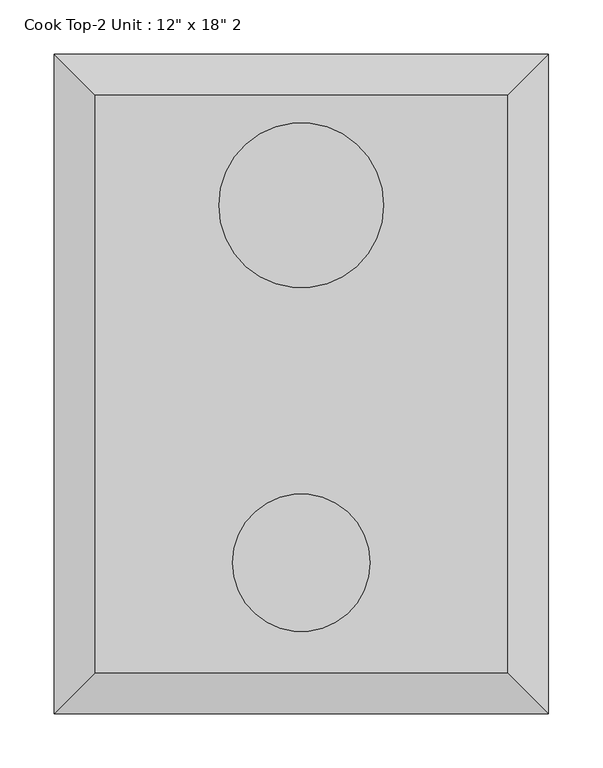
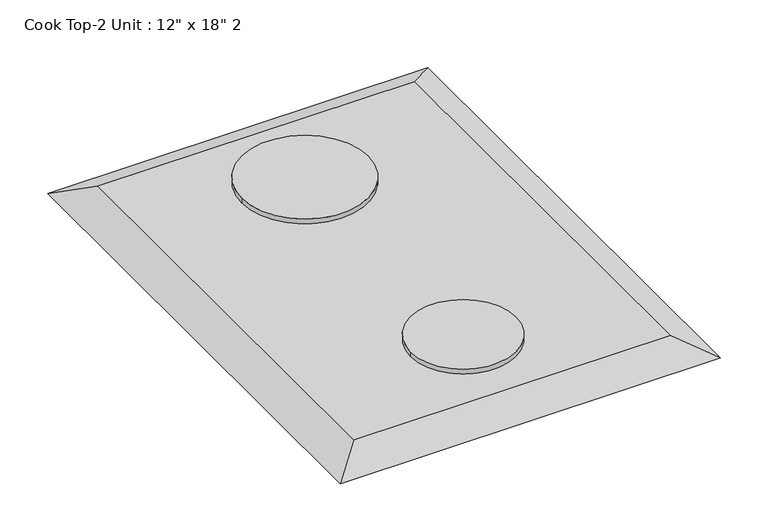
"""IFC4 building model written with IfcOpenShell, lengths in millimetres: proxy geometry."""

from ifc_helpers import new_model, si_unit, point, frame, frame_2d, origin, place, context, project, spatial, circle_curve, trimmed, segment, composite_curve, outline, extrude, faceted_brep, source, transform, mapped, element, save


def proxy_3c1fa1d0(model_context):
    return source(origin(), model_context, "Body", "SolidModel", [
        faceted_brep([(266.7, 296.9247956, 933.45), (-114.3, 296.9247956, 933.45), (-114.3, -236.4752044, 933.45), (266.7, -236.4752044, 933.45), (304.8, 335.0247956, 914.4), (304.8, -274.5752044, 914.4), (-152.4, -274.5752044, 914.4), (-152.4, 335.0247956, 914.4)], [[[0, 1, 2, 3]], [[4, 5, 6, 7]], [[4, 7, 1, 0]], [[7, 6, 2, 1]], [[6, 5, 3, 2]], [[5, 4, 0, 3]]]),
        extrude(outline(composite_curve([segment(trimmed(circle_curve(frame_2d((76.2, 195.3247956)), 76.2), [point((152.4, 195.3247956))], [point((0.0, 195.3247956))], False, "CARTESIAN"), True, "CONTINUOUS"), segment(trimmed(circle_curve(frame_2d((76.2, 195.3247956)), 76.2), [point((0.0, 195.3247956))], [point((152.4, 195.3247956))], False, "CARTESIAN"), True, "CONTINUOUS")], self_intersect=False)), frame((0.0, 0.0, 933.45), z_axis=(0.0, 0.0, 1.0), x_axis=(1.0, 0.0, 0.0)), (0.0, 0.0, 1.0), 6.35),
        extrude(outline(composite_curve([segment(trimmed(circle_curve(frame_2d((76.2, -134.8752044)), 63.5), [point((139.7, -134.8752044))], [point((12.7, -134.8752044))], False, "CARTESIAN"), True, "CONTINUOUS"), segment(trimmed(circle_curve(frame_2d((76.2, -134.8752044)), 63.5), [point((12.7, -134.8752044))], [point((139.7, -134.8752044))], False, "CARTESIAN"), True, "CONTINUOUS")], self_intersect=False)), frame((0.0, 0.0, 933.45), z_axis=(0.0, 0.0, 1.0), x_axis=(1.0, 0.0, 0.0)), (0.0, 0.0, 1.0), 6.35),
    ])


if __name__ == "__main__":
    model = new_model("IFC4")
    model_context = context("Model", 3, world=origin())
    ifc_project = project(units=[si_unit("LENGTHUNIT", "METRE", prefix="MILLI")], contexts=[model_context])
    site = spatial("IfcSite", under=ifc_project)
    building = spatial("IfcBuilding", under=site)
    placement = place(None, origin())
    proxy_shape = proxy_3c1fa1d0(model_context)
    element("IfcBuildingElementProxy", 1, Name="Cook Top-2 Unit : 12\" x 18\" 2", ObjectType="Cook Top-2 Unit : 12\" x 18\" 2", at=placement, inside=building, context=model_context, shape_type="MappedRepresentation", body=[
        mapped(proxy_shape, transform((0.0, 0.0, 0.0), x_axis=(1.0, 0.0, 0.0), y_axis=(0.0, 1.0, 0.0), z_axis=(0.0, 0.0, 1.0))),
    ])
    save(model, "model.ifc")

# Revit data of these elements
# Type "Cook Top-2 Unit : 12\" x 18\" 2"
#   Assembly Code = "E1090400"
#   Counter Height = 3' - 0"
#   Depth = 2' - 0"
#   Width = 1' - 6"
#   Burner Material = Metal - Chrome
#   Cooktop Material = Metal - Steel, Polished
#   Default Elevation = 0
# Element 1 (IfcBuildingElementProxy, "Cook Top-2 Unit : 12\" x 18\" 2")
#   Materials on its faces: "Metal - Steel, Polished", "Metal - Chrome"
# Materials
#   "Metal - Chrome": colour RGB 17 17 17, transparency 0
#   "Metal - Steel, Polished": colour RGB 127 127 127, transparency 0
